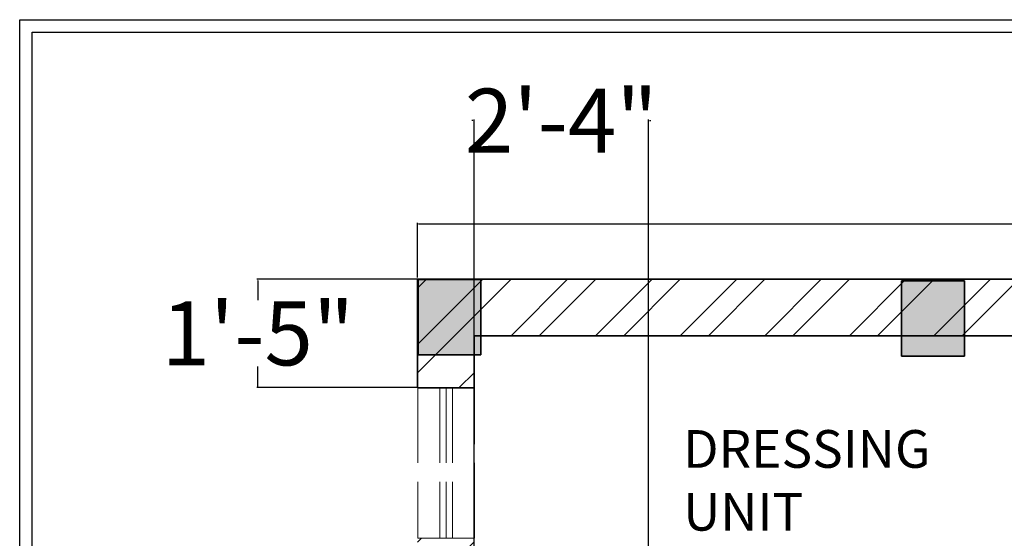
# Model space of a CAD drawing. Units: inches. Extents: x 1812 to 2791, y 2306 to 2959.
# Tile 3 of 8: x 1827 to 1984, y 2856 to 2939. Entities that reach past the tile are written whole.
import ezdxf

# ---------------------------------------------------------------- set-up
doc = ezdxf.new("R2010")
doc.units = ezdxf.units.IN
doc.linetypes.add('ACAD_ISO02W100', pattern=[15, 12, -3])
doc.layers.get('Defpoints').update_dxf_attribs({"lineweight": 50})
for name, color, linetype, lineweight in [('A-ANNO-DIMS', 2, 'Continuous', 18), ('A-ANNO-TTLB', 7, 'Continuous', 25), ('A-AREA-IDEN', 7, 'Continuous', 18), ('A-COLS', 7, 'Continuous', 35), ('A-FLOR-CASE', 8, 'Continuous', 18), ('A-GLAZ-VENT', 6, 'ACAD_ISO02W100', 13), ('A-WALL-PATT', 8, 'Continuous', 13), ('WALL', 7, 'Continuous', 35)]:
    doc.layers.add(name, color=color, linetype=linetype, lineweight=lineweight)
doc.styles.get("Standard").update_dxf_attribs({"font": 'arial.ttf'})
doc.dimstyles.get("Standard").update_dxf_attribs({"dimtxt": 10.18, "dimasz": 0.18, "dimexe": 0.18, "dimexo": 0.0625, "dimgap": 0.09, "dimtad": 0, "dimtih": 1, "dimtoh": 1, "dimdec": 0, "dimzin": 0, "dimdsep": 46, "dimlunit": 3, "dimtxsty": 'Standard', "dimcen": 0.09, "dimadec": 0, "dimazin": 0, "dimtfac": 1, "dimtdec": 0, "dimtofl": 0, "dimtmove": 0, "dimatfit": 3, "dimfxl": 1, "dimtolj": 1, "dimtzin": 0, "dimarcsym": 0})

# ---------------------------------------------------------------- blocks, each defined once
blk = doc.blocks.new('*D14')
at = {"layer": 'A-ANNO-DIMS', "color": 0, "lineweight": -2, "transparency": 16777216}
for p, q in [((1890.367596134611, 2897.88570642368), (1890.367596134611, 2906.587838465212)), ((1890.547596134611, 2906.407838465212), (2001.608675586698, 2906.407838465212)), ((2130.300191600858, 2906.407838465212), (2019.239112148772, 2906.407838465212)), ((2130.480191600858, 2897.88570642368), (2130.480191600858, 2906.587838465212))]:
    blk.add_line(p, q, dxfattribs=at)
at = {"layer": 'A-ANNO-DIMS', "color": 0, "transparency": 16777216}
for points in [[(1890.547596134611, 2906.437838465212), (1890.547596134611, 2906.377838465212), (1890.367596134611, 2906.407838465212)], [(2130.300191600858, 2906.437838465212), (2130.300191600858, 2906.377838465212), (2130.480191600858, 2906.407838465212)]]:
    blk.add_solid(points, dxfattribs=at)
at = {"layer": 'Defpoints', "color": 0, "transparency": 16777216}
for p in [(2130.480191600858, 2906.407838465212), (1890.367596134611, 2897.82320642368), (2130.480191600858, 2897.82320642368)]:
    blk.add_point(p, dxfattribs=at)
at = {"layer": 'A-ANNO-DIMS', "color": 0, "transparency": 16777216, "insert": (2010.423893867735, 2906.407838465212), "char_height": 10.18, "attachment_point": 5}
blk.add_mtext("\\A1;20'", dxfattribs=at)
blk = doc.blocks.new('COL')
at = {"transparency": 33554687}
h = blk.add_hatch(color=256, dxfattribs=at)
h.dxf.hatch_style = 1
h.paths.add_polyline_path([(2424.397880689844, 2829.240948453883), (2424.397880689844, 2839.240948453883), (2412.397880689843, 2839.240948453883), (2412.397880689843, 2829.240948453883)])
for p, q in [((2412.397880689843, 2839.240948453883), (2424.397880689844, 2839.240948453883)), ((2412.397880689843, 2839.240948453883), (2412.397880689843, 2829.240948453882)), ((2424.397880689844, 2839.240948453883), (2424.397880689844, 2829.240948453883)), ((2412.397880689843, 2829.240948453883), (2424.397880689844, 2829.240948453883))]:
    blk.add_line(p, q)
blk = doc.blocks.new('VENT-24x9')
for p, q in [((3.499863851171994, 23.99973038050894), (3.499863851171994, -0.0002696194910641)), ((4.499863851171994, 23.99973038050894), (4.499863851171994, -0.0002696194910641)), ((5.499863851171994, 23.99973038050894), (5.499863851171994, -0.0002696194910641))]:
    blk.add_line(p, q)
blk.add_lwpolyline([(-0.0001361485951747, -0.0002696194910641), (8.999863851404825, -0.0002696194910641), (8.999863851171995, 23.99973038050894), (-0.0001361488280054, 23.99973038050894)], close=True)
blk = doc.blocks.new('SHEET-FRAME-RESIDENCE')
blk.add_lwpolyline([(0.000131823559741, 632.8005012919775), (378.7609620870107, 632.8005012919775), (378.7609620870107, 0.0003856501880364), (0.000131823559741, 0.0003856501880364)], close=True)
blk.add_lwpolyline([(2.00013182355974, 71.32450104412055), (2.00013182355974, 630.8005012919775), (376.7609620870107, 630.8005012919775), (376.7609620870107, 71.32450104412055)])
blk = doc.blocks.new('*D51')
at = {"layer": 'A-ANNO-DIMS', "color": 0, "lineweight": -2, "transparency": 16777216}
for p, q in [((2010.613726114925, 2887.157800411407), (1995.646226114926, 2887.157800411407)), ((1995.826226114926, 2886.977800411407), (1995.826226114926, 2854.714874081257)), ((1995.826226114926, 2811.737800411407), (1995.826226114926, 2844.000726741557)), ((2010.613726114925, 2811.557800411407), (1995.646226114926, 2811.557800411407))]:
    blk.add_line(p, q, dxfattribs=at)
at = {"layer": 'A-ANNO-DIMS', "color": 0, "transparency": 16777216}
for points in [[(1995.796226114926, 2886.977800411407), (1995.856226114926, 2886.977800411407), (1995.826226114926, 2887.157800411407)], [(1995.796226114926, 2811.737800411407), (1995.856226114926, 2811.737800411407), (1995.826226114926, 2811.557800411407)]]:
    blk.add_solid(points, dxfattribs=at)
at = {"layer": 'Defpoints', "color": 0, "transparency": 16777216}
for p in [(1995.826226114926, 2887.157800411407), (2010.676226114925, 2887.157800411407), (2010.676226114925, 2811.557800411407)]:
    blk.add_point(p, dxfattribs=at)
at = {"layer": 'A-ANNO-DIMS', "color": 0, "transparency": 16777216, "insert": (1995.826226114926, 2849.357800411406), "char_height": 10.18, "attachment_point": 5}
blk.add_mtext('\\A1;6\'-3 1/2" TYP.', dxfattribs=at)
blk = doc.blocks.new('*D75')
at = {"layer": 'A-ANNO-DIMS', "color": 0, "lineweight": -2, "transparency": 16777216}
for p, q in [((1899.206542, 2922.852944), (1899.026542, 2922.852944)), ((1899.386542, 2838.665444), (1899.386542, 2923.032944)), ((1927.158944, 2838.665444), (1927.158944, 2923.032944)), ((1927.338944, 2922.852944), (1927.518944, 2922.852944))]:
    blk.add_line(p, q, dxfattribs=at)
at = {"layer": 'A-ANNO-DIMS', "color": 0, "transparency": 16777216}
for points in [[(1899.206542, 2922.882944000001), (1899.206542, 2922.822944), (1899.386542, 2922.852944)], [(1927.338944, 2922.882944000001), (1927.338944, 2922.822944), (1927.158944, 2922.852944)]]:
    blk.add_solid(points, dxfattribs=at)
at = {"layer": 'Defpoints', "color": 0, "transparency": 16777216}
for p in [(1927.158944, 2922.852944), (1899.386542, 2838.602944), (1927.158944, 2838.602944)]:
    blk.add_point(p, dxfattribs=at)
at = {"layer": 'A-ANNO-DIMS', "color": 0, "transparency": 16777216, "insert": (1913.272743, 2922.852944), "char_height": 10.18, "attachment_point": 5}
blk.add_mtext('\\A1;2\'-4"', dxfattribs=at)
blk = doc.blocks.new('*D76')
at = {"layer": 'A-ANNO-DIMS', "color": 0, "lineweight": -2, "transparency": 16777216}
for p, q in [((1890.324042000001, 2897.602944000001), (1864.780736000002, 2897.602944000001)), ((1864.960736000002, 2897.422944000001), (1864.960736000002, 2894.269970015008)), ((1864.960736000002, 2880.541730000001), (1864.960736000002, 2883.694703984994)), ((1890.364364000001, 2880.361730000001), (1864.780736000002, 2880.361730000001))]:
    blk.add_line(p, q, dxfattribs=at)
at = {"layer": 'A-ANNO-DIMS', "color": 0, "transparency": 16777216}
for points in [[(1864.930736000002, 2897.422944000001), (1864.990736000002, 2897.422944000001), (1864.960736000002, 2897.602944000001)], [(1864.930736000002, 2880.541730000001), (1864.990736000002, 2880.541730000001), (1864.960736000002, 2880.361730000001)]]:
    blk.add_solid(points, dxfattribs=at)
at = {"layer": 'Defpoints', "color": 0, "transparency": 16777216}
for p in [(1890.386542000001, 2897.602944000001), (1864.960736000002, 2880.361730000001), (1890.426864000001, 2880.361730000001)]:
    blk.add_point(p, dxfattribs=at)
at = {"layer": 'A-ANNO-DIMS', "color": 0, "transparency": 16777216, "insert": (1864.960736000002, 2888.982337000001), "char_height": 10.18, "attachment_point": 5}
blk.add_mtext('\\A1;1\'-5"', dxfattribs=at)

msp = doc.modelspace()

# ---------------------------------------------------------------- hatches: boundary and pattern name
at = {"layer": 'A-WALL-PATT'}
h = msp.add_hatch(dxfattribs=at)
h.set_pattern_fill('ANSI32', color=256)
h.set_pattern_definition([(45, (0, 0), (-6.735192090801865, 6.735192090801866), []), (45, (4.49013, 0), (-6.735192090801865, 6.735192090801866), [])])
h.paths.add_polyline_path([(2130.386541883867, 2417.602943720933), (2119.693765675914, 2417.602943720932), (2119.693765675914, 2768.55867658318), (2121.386541883867, 2768.55867658318), (2121.386541883867, 2801.624379255592), (2121.320110177716, 2849.363725604599), (2121.320110177716, 2801.624379255592), (2130.386541883867, 2801.624379255592)])
h.paths.add_polyline_path([(2023.386541883867, 2426.602943720928), (1899.386541883867, 2426.602943720922), (1899.386541883867, 2453.602943720933), (1951.802463468582, 2453.602943720933), (1951.802463468583, 2457.602943720932), (1899.386541883867, 2457.602943720932), (1899.386541883867, 2590.602943720933), (1959.931736449602, 2590.602943720933), (1959.931736449602, 2594.602943720933), (1899.386541883867, 2594.602943720933), (1899.386541883867, 2634.525457409657), (1890.386541883867, 2634.525457409656), (1890.386541883867, 2417.602943720933), (2023.386541883867, 2417.602943720933)])
h.paths.add_polyline_path([(2119.693765675914, 2426.602943720933), (2112.386541883867, 2426.602943720932), (2112.386541883867, 2417.602943720932), (2119.693765675914, 2417.602943720933)])
h.paths.add_polyline_path([(1899.386541883867, 2740.602943720932), (1941.386541883867, 2740.602943720932), (1941.386541883866, 2744.602943720933), (1899.386541883867, 2744.602943720932), (1899.386541883867, 2772.941372394735), (1890.386541883867, 2772.941372394735), (1890.386541883867, 2682.525457409656), (1899.210735520098, 2682.525457409656), (1899.210735520098, 2682.638517261234)])
h.paths.add_polyline_path([(1975.386541883867, 2838.602943720933), (1899.386541883867, 2838.602943720932), (1899.386541883866, 2856.334456704745), (1890.386541883867, 2856.334456704745), (1890.386541883867, 2796.94720306846), (1899.386541883867, 2796.94720306846), (1899.386541883867, 2834.602943720933), (1971.386541883867, 2834.602943720933), (1971.386541883867, 2740.602943720933), (1975.386541883867, 2740.602943720933)])
h.paths.add_polyline_path([(2119.693765675914, 2897.602943720933), (1890.386541883867, 2897.602943720933), (1890.386541883867, 2880.361730380509), (1899.386541883866, 2880.361730380509), (1899.386541883867, 2888.602943720933), (2119.693765675914, 2888.602943720933)])
h.paths.add_polyline_path([(2130.386541883867, 2897.602943720933), (2119.693765675914, 2897.602943720933), (2119.693765675914, 2888.602943720933), (2121.386541883867, 2888.602943720933), (2121.386541883867, 2849.624379255592), (2130.386541883867, 2849.624379255592)])

# ---------------------------------------------------------------- linework, layer by layer
at = {"layer": 'A-FLOR-CASE'}
msp.add_line((1927.158943641966, 2888.602943720933), (1927.158943641966, 2838.602943720933), dxfattribs=at)
at = {"layer": 'WALL'}
for p, q in [((1890.386541883867, 2897.602943720933), (2130.386541883867, 2897.602943720933)), ((1890.386541883867, 2880.334456704744), (1890.386541883867, 2897.602943720933)), ((1899.386541883867, 2888.602943720933), (2121.386541883867, 2888.602943720933)), ((1899.386541883866, 2880.334456704744), (1899.386541883867, 2888.602943720933)), ((1890.386541883867, 2880.334456704744), (1899.386541883866, 2880.334456704744))]:
    msp.add_line(p, q, dxfattribs=at)

# ---------------------------------------------------------------- block references
at = {"layer": 'A-ANNO-TTLB'}
msp.add_blockref('SHEET-FRAME-RESIDENCE', (1827.027, 2306.124), dxfattribs=at)
at = {"layer": 'A-COLS', "rotation": 270}
for p in [(-938.7622940082643, 5309.941982927579), (-861.7732573554129, 5309.762172758523)]:
    msp.add_blockref('COL', p, dxfattribs=at)
at = {"layer": 'A-GLAZ-VENT'}
msp.add_blockref('VENT-24x9', (1890.427, 2856.362), dxfattribs=at)

# ---------------------------------------------------------------- texts
at = {"layer": 'A-AREA-IDEN', "insert": (1932.690324151171, 2873.586660576948), "char_height": 6, "attachment_point": 1}
msp.add_mtext_dynamic_manual_height_columns('DRESSING\\PUNIT', width=184.43951469184, gutter_width=12.5, heights=[0], dxfattribs=at)

# ---------------------------------------------------------------- dimensions: what is measured, and where the dimension line sits
at = {"layer": 'A-ANNO-DIMS'}
for base, p1, p2, override, picture, middle in [((1927.158944, 2922.852944), (1899.386542, 2838.602944), (1927.158944, 2838.602944), {"dimdec": 1, "dimlfac": 1, "dimrnd": 0, "dimzin": 1, "dimdsep": 46, "dimlunit": 4, "dimfrac": 2}, '*D75', (1913.272743, 2922.852944)), ((2130.480191600858, 2906.407838465212), (1890.367596134611, 2897.82320642368), (2130.480191600858, 2897.82320642368), {"dimclrd": 0, "dimclre": 0, "dimclrt": 0}, '*D14', (2010.423893867735, 2906.407838465212))]:
    dim = msp.add_linear_dim(base=base, p1=p1, p2=p2, dimstyle='Standard', override=override, dxfattribs=at)
    dim.commit()
    dim.dimension.update_dxf_attribs({"geometry": picture, "text_midpoint": middle})
dim = msp.add_linear_dim(base=(1864.960736000002, 2880.361730000001), p1=(1890.386542, 2897.602944), p2=(1890.426864, 2880.36173), angle=90, dimstyle='Standard', override={"dimdec": 1, "dimlfac": 1, "dimrnd": 0, "dimzin": 1, "dimdsep": 46, "dimlunit": 4, "dimfrac": 2}, dxfattribs=at)
dim.commit()
dim.dimension.update_dxf_attribs({"geometry": '*D76', "text_midpoint": (1864.960736000002, 2888.982337000001)})
dim = msp.add_linear_dim(base=(1995.826226114926, 2887.157800411407), p1=(2010.676226114924, 2811.557800411406), p2=(2010.676226114924, 2887.157800411406), angle=90, text='<> TYP.', dimstyle='Standard', override={"dimdec": 1, "dimlfac": 1, "dimrnd": 0, "dimzin": 1, "dimdsep": 46, "dimlunit": 4, "dimfrac": 2}, dxfattribs=at)
dim.commit()
dim.dimension.update_dxf_attribs({"geometry": '*D51', "text_midpoint": (1995.826226114926, 2849.357800411406)})

doc.saveas('drawing.dxf')
